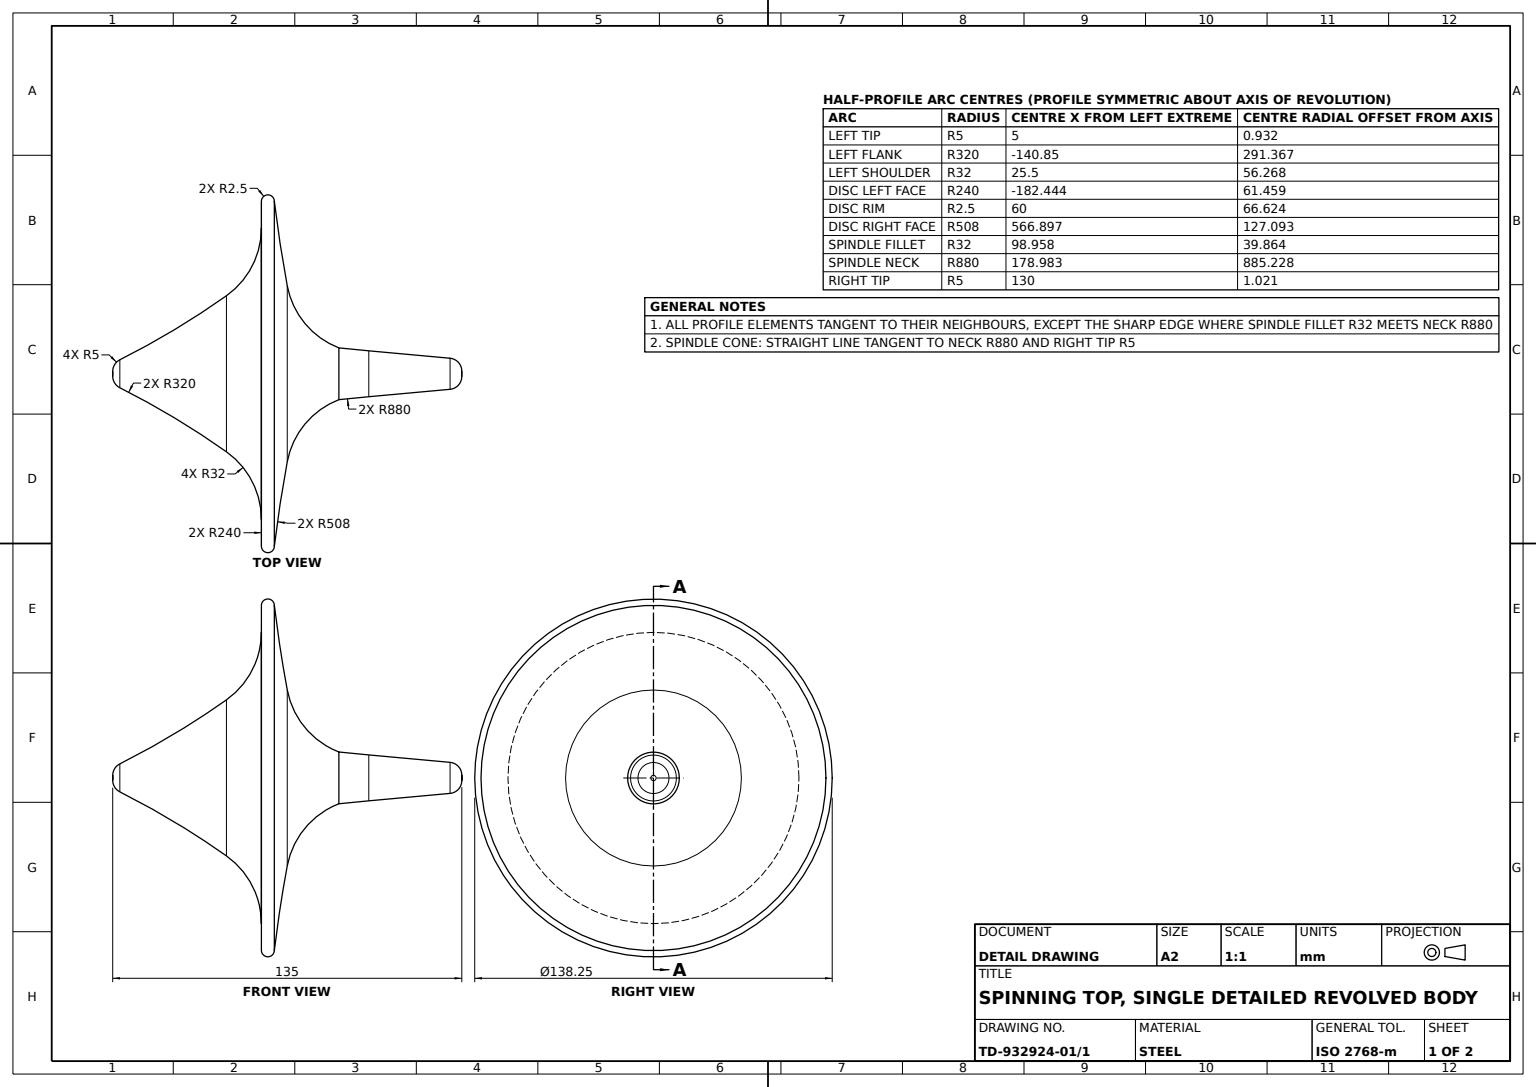
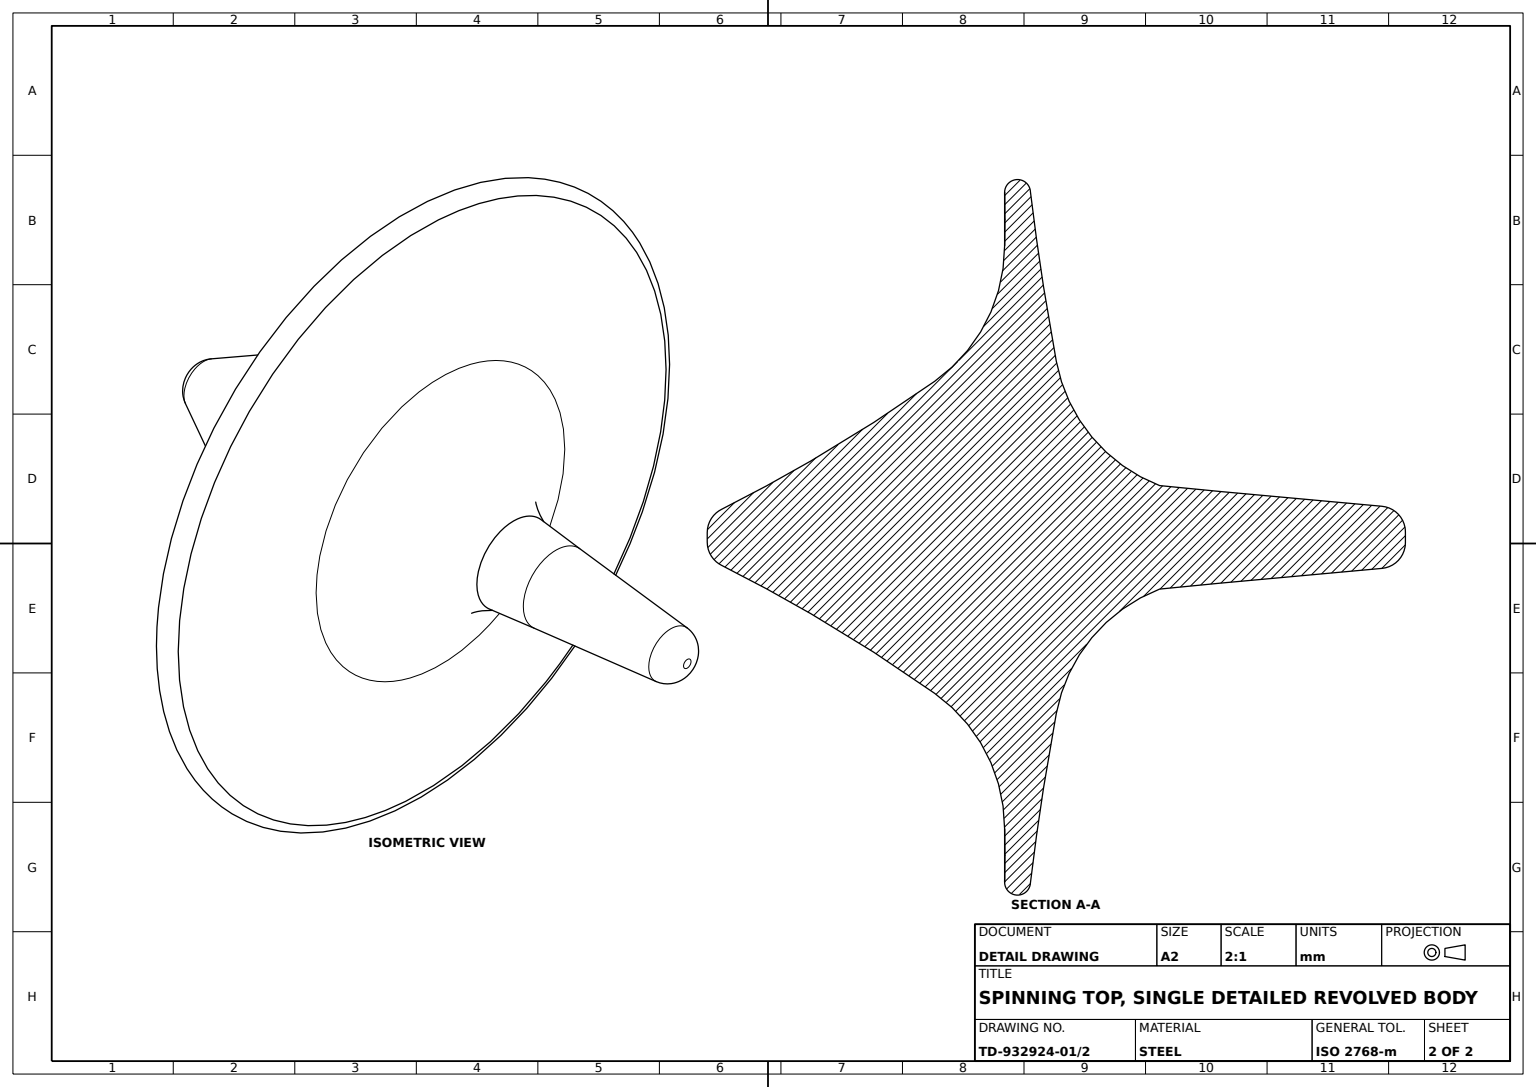
from build123d import *


with BuildPart() as part:
    # Top Half Profile → Spinning Top Revolve (revolve)
    with BuildSketch(Plane.XY, mode=Mode.PRIVATE) as spinning_top_revolve_sk:
        with BuildLine():
            ThreePointArc((66.699946845, -5), (69.123205901, -7.563423043), (66.570796819, -9.998280333))
            ThreePointArc((66.570796819, -9.998280333), (61.41938821, -9.943848556), (56.267998059, -10))
            ThreePointArc((56.267998059, -10), (41.561999586, -13.579345382), (30.145866595, -23.516649444))
            ThreePointArc((30.145866595, -23.516649444), (16.997479936, -43.6647974), (5.4, -64.743848539))
            ThreePointArc((5.4, -64.743848539), (3.55671587, -66.755540077), (0.931762793, -67.5))
            Line((0.931762793, -67.5), (0, -67.5))
            Line((0, -67.5), (0, 67.5))
            Line((0, 67.5), (1.02149392, 67.5))
            ThreePointArc((1.02149392, 67.5), (4.389313376, 66.19564502), (6, 62.963116845))
            Line((6, 62.963116845), (8.867384456, 31.532882589))
            ThreePointArc((8.867384456, 31.532882589), (9.414586997, 25.746129421), (10, 19.963116845))
            ThreePointArc((10, 19.963116845), (19.400534743, 6.856436897), (34, 0))
            ThreePointArc((34, 0), (50.309263809, -2.766240437), (66.699946845, -5))
        make_face()
    revolve(spinning_top_revolve_sk.sketch.rotate(Axis((0, 67.5, 0), (0, -1, 0)), 90), axis=Axis((0, 67.5, 0), (0, -1, 0)))


solid = part.part
